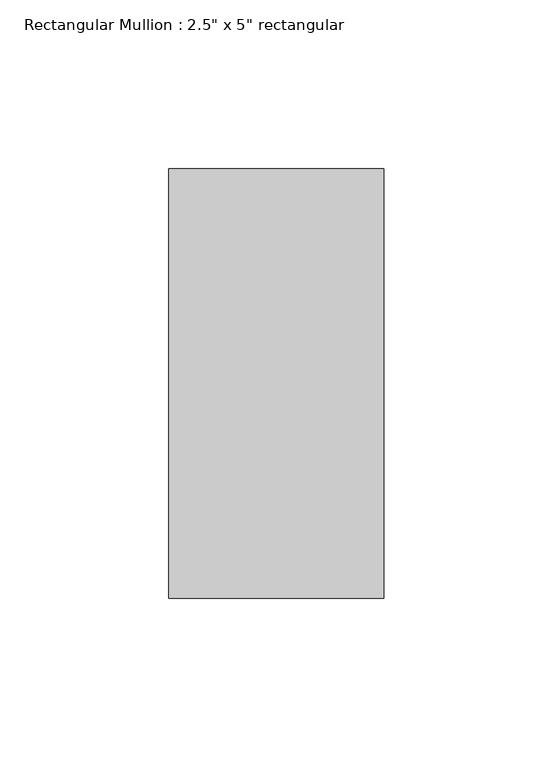
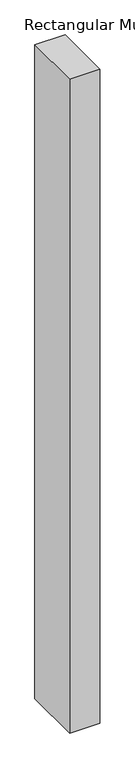
"""IFC4 building model written with IfcOpenShell, lengths in millimetres: member geometry."""

from ifc_helpers import new_model, si_unit, frame, origin, place, context, project, spatial, polyline, outline, extrude, source, transform, mapped, element, save


def member_6045db05(model_context):
    return source(origin(), model_context, "Body", "SweptSolid", [
        extrude(outline(polyline([(31.75, 63.5), (31.75, -63.5), (-31.75, -63.5), (-31.75, 63.5), (31.75, 63.5)])), frame((0.0, 0.0, -1456.6512079), z_axis=(0.0, 0.0, 1.0), x_axis=(1.0, 0.0, 0.0)), (0.0, 0.0, 1.0), 1456.6512079),
    ])


if __name__ == "__main__":
    model = new_model("IFC4")
    model_context = context("Model", 3, world=origin())
    ifc_project = project(units=[si_unit("LENGTHUNIT", "METRE", prefix="MILLI")], contexts=[model_context])
    site = spatial("IfcSite", under=ifc_project)
    building = spatial("IfcBuilding", under=site)
    placement = place(None, origin())
    member_shape = member_6045db05(model_context)
    element("IfcMember", 1, ObjectType="Rectangular Mullion : 2.5\" x 5\" rectangular", at=placement, inside=building, context=model_context, shape_type="MappedRepresentation", body=[
        mapped(member_shape, transform((0.0, 0.0, 0.0), x_axis=(1.0, 0.0, 0.0), y_axis=(0.0, 1.0, 0.0), z_axis=(0.0, 0.0, 1.0))),
    ])
    save(model, "model.ifc")

# Revit data of these elements
# Type "Rectangular Mullion : 2.5\" x 5\" rectangular"
#   built-in parameter 1007304 = 0.416667 (stored number, unit not read)
#   built-in parameter 1007301 = 0.104167 (stored number, unit not read)
#   built-in parameter 1007300 = 0.104167 (stored number, unit not read)
# Element 1 (IfcMember, "Rectangular Mullion : 2.5\" x 5\" rectangular")
#   Materials on its faces: "Aluminum"
# Materials
#   "Aluminum": class "Metal", colour RGB 247 247 247, transparency 0, Description = "Aluminum 6061", Cost = 0
